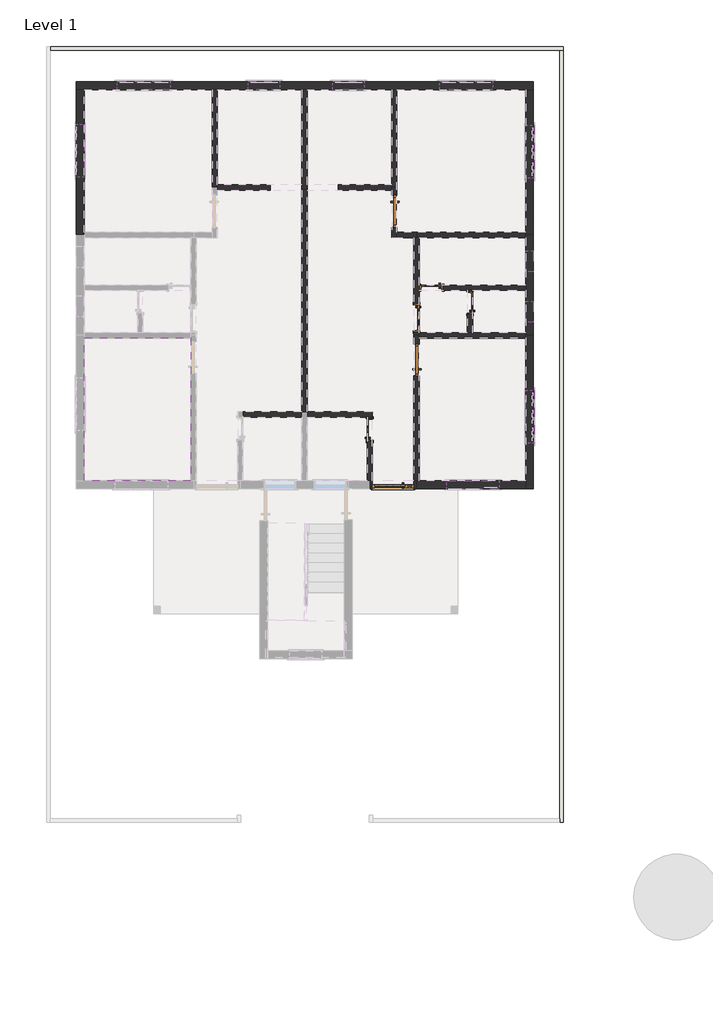
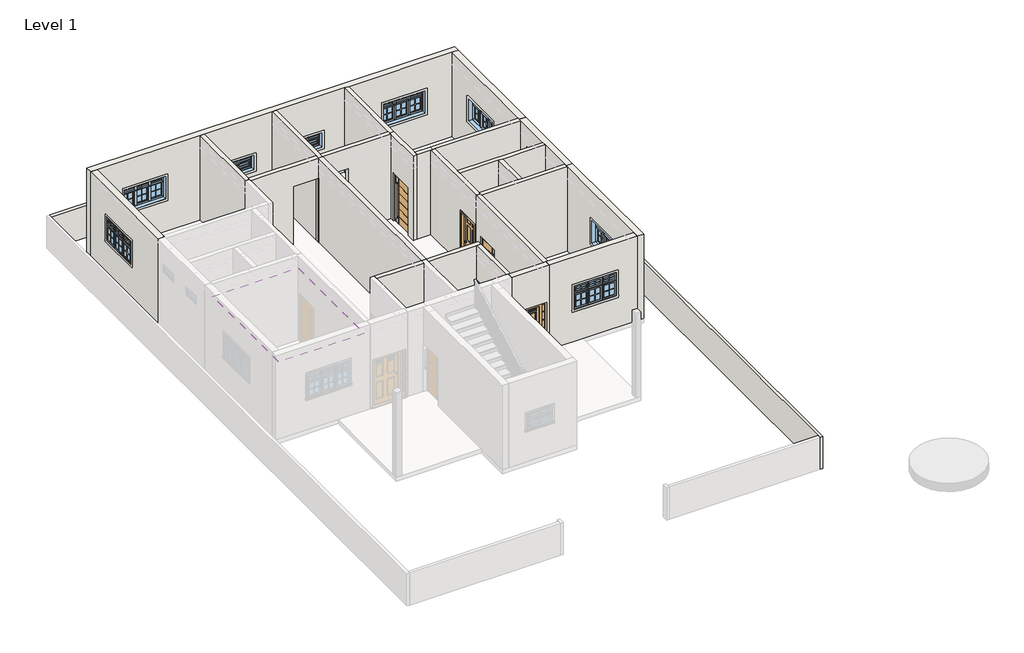
# One storey, part 2 of 4: 25 walls, 10 windows, 7 doors, 1 covering.
# Revit data of these elements (continued)
# Element 38 (IfcWindow, "M_Window-Casement-Triple-Awning-Triple : 5'") (continued)
#   Interior Wall Closure = 0' - 2.15551"
#   Frame Extension = 0' - 0 1/4"
#   Exterior Wall Closure = 0' - 1 1/4"
#   Interior Trim Visibility = yes
#   Exterior Trim Visibility = yes
#   Phase Created = New Construction
#   Materials on its faces: "Wood - Stained", "Glass", "Clad - White"
# Element 39 (IfcWindow, "M_Window-Casement-Triple-Awning-Triple : 5'")
#   Mark = "2"
#   Window Inset = 0' - 0"
#   Interior Wall Closure = 0' - 2.15551"
#   Frame Extension = 0' - 0 1/4"
#   Exterior Wall Closure = 0' - 1 1/4"
#   Interior Trim Visibility = yes
#   Exterior Trim Visibility = yes
#   Phase Created = New Construction
#   Materials on its faces: "Wood - Stained", "Glass", "Clad - White"
# Element 40 (IfcWindow, "M_Window-Casement-Triple-Awning-Triple : 5'")
#   Mark = "3"
#   Window Inset = 0' - 0"
#   Interior Wall Closure = 0' - 2.15551"
#   Frame Extension = 0' - 0 1/4"
#   Exterior Wall Closure = 0' - 1 1/4"
#   Interior Trim Visibility = yes
#   Exterior Trim Visibility = yes
#   Phase Created = New Construction
#   Materials on its faces: "Wood - Stained", "Glass", "Clad - White"
# Element 41 (IfcWindow, "M_Window-Casement-Triple-Awning-Triple : 5'")
#   Mark = "4"
#   Window Inset = 0' - 0"
#   Interior Wall Closure = 0' - 2.15551"
#   Frame Extension = 0' - 0 1/4"
#   Exterior Wall Closure = 0' - 1 1/4"
#   Interior Trim Visibility = yes
#   Exterior Trim Visibility = yes
#   Phase Created = New Construction
#   Materials on its faces: "Wood - Stained", "Glass", "Clad - White"
# Element 42 (IfcWindow, "M_Window-Casement-Triple-Awning-Triple : 5'")
#   Mark = "5"
#   Window Inset = 0' - 0"
#   Interior Wall Closure = 0' - 2.15551"
#   Frame Extension = 0' - 0 1/4"
#   Exterior Wall Closure = 0' - 1 1/4"
#   Interior Trim Visibility = yes
#   Exterior Trim Visibility = yes
#   Phase Created = New Construction
#   Materials on its faces: "Wood - Stained", "Glass", "Clad - White"
# Element 43 (IfcWindow, "M_Window-Casement-Triple-Awning-Triple : 5'")
#   Mark = "6"
#   Window Inset = 0' - 0"
#   Interior Wall Closure = 0' - 2.15551"
#   Frame Extension = 0' - 0 1/4"
#   Exterior Wall Closure = 0' - 1 1/4"
#   Interior Trim Visibility = yes
#   Exterior Trim Visibility = yes
#   Phase Created = New Construction
#   Materials on its faces: "Wood - Stained", "Glass", "Clad - White"
# Materials
#   "Default": colour RGB 127 127 127, transparency 0, Cost = 0
#   "Acoustic Ceiling Tile 24 x 48": class "Generic", colour RGB 229 229 229, transparency 0, Description = "Acoustic Ceiling Tile 24 x 48", Cost = 0
#   "Door - Glazing": colour RGB 0 0 255, transparency 0.75
#   "Door - Panel": class "Wood", colour RGB 210 159 95, transparency 0, Cost = 0
#   "Door - Handle": colour RGB 246 240 166, transparency 0
#   "Cherry": class "Wood", colour RGB 226 177 128, transparency 0, Description = "Prunus Serotina", Cost = 0
#   "Aluminum": class "Metal", colour RGB 247 247 247, transparency 0, Description = "Aluminum 6061", Cost = 0
#   "Glass": class "Glass", colour RGB 0 128 192, transparency 0.75, Description = "Soda Lime Glass", Cost = 0
#   "Sash": class "Wood", colour RGB 224 178 126, transparency 0, Cost = 0
#   "Wood - Stained": class "Wood", colour RGB 224 178 126, transparency 0, Cost = 0
#   "Clad - White": class "Wood", colour RGB 242 242 238, transparency 0, Cost = 0
#   "LVW1": class "Generic", colour RGB 120 120 120, transparency 0, Cost = 0
#   "Default Wall": colour RGB 128 128 128, transparency 0, Cost = 0
#   "BED ROOM WALL 1": class "Generic", colour RGB 120 120 120, transparency 0, Cost = 0
#   "BED ROOM WALL 2": class "Generic", colour RGB 120 120 120, transparency 0, Cost = 0
#   "BAW1": class "Generic", colour RGB 120 120 120, transparency 0, Cost = 0
#   "BAW2": class "Generic", colour RGB 120 120 120, transparency 0, Cost = 0
